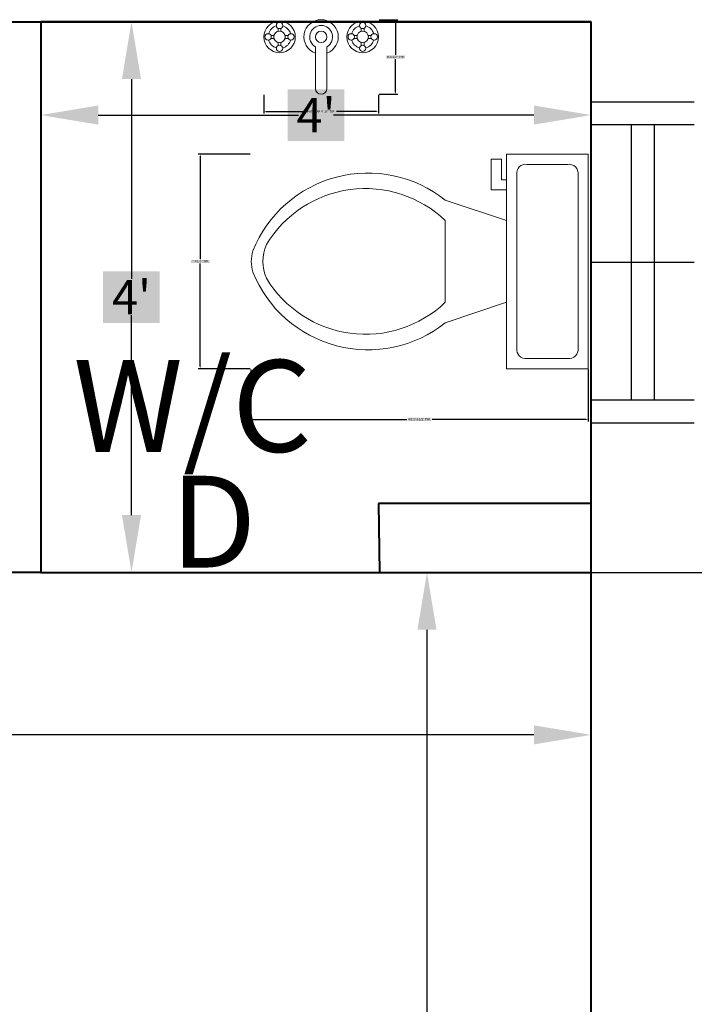
# Model space of a CAD drawing. Units: inches. Extents: x -301 to 715, y -607 to 364.
# Tile 93 of 141: x 74 to 133, y -168 to -83. Entities that reach past the tile are written whole.
import ezdxf

# ---------------------------------------------------------------- set-up
doc = ezdxf.new("R2010")
doc.units = ezdxf.units.IN
doc.header["$MEASUREMENT"] = 0
for name, color, linetype, lineweight in [('A-ANNO-DIMS', 2, 'Continuous', 18), ('A-ANNO-TEXT', 4, 'Continuous', 18), ('A-AREA-IDEN', 220, 'Continuous', 25), ('A-FLOR-FIXT', 9, 'Continuous', 18), ('A-GLAZ', 2, 'Continuous', 25), ('A-WALL', 3, 'Continuous', 40)]:
    doc.layers.add(name, color=color, linetype=linetype, lineweight=lineweight)
doc.styles.get("Standard").update_dxf_attribs({"font": 'arial.ttf'})
doc.dimstyles.get("Standard").update_dxf_attribs({"dimtxt": 0.18, "dimasz": 0.18, "dimexe": 0.18, "dimexo": 0.0625, "dimgap": 0.09, "dimtad": 0, "dimtih": 1, "dimtoh": 1, "dimdec": 1, "dimzin": 0, "dimdsep": 46, "dimlunit": 4, "dimtxsty": 'Standard', "dimcen": 0.09, "dimclrd": 3, "dimclre": 4, "dimclrt": 6, "dimadec": 0, "dimazin": 0, "dimtfac": 1, "dimtdec": 1, "dimtofl": 0, "dimtmove": 0, "dimatfit": 3, "dimfxl": 1, "dimtfill": 2, "dimtfillclr": 51, "dimtolj": 1, "dimtzin": 0, "dimarcsym": 0})

# ---------------------------------------------------------------- blocks, each defined once
blk = doc.blocks.new('Toilet - top')
for p, q in [((9.5, -6), (9.5, -2)), ((-10, -8.5), (-8, -8.5)), ((-10, -9.5), (-10, -8.5)), ((-8, -8.5), (-8, -8)), ((-7, -8), (-7, -9.5)), ((-4, -8), (-6, -14)), ((4, -8), (6, -14)), ((-7, -9.5), (-10, -9.5)), ((4, -14), (-4, -14))]:
    blk.add_line(p, q)
blk.add_lwpolyline([(10.5, -8), (10.5, 0), (-10.5, 0), (-10.5, -8)], close=True)
for points in [[(8.5, -1), (-8.5, -1)], [(-9.5, -2), (-9.5, -6)], [(-8.5, -7), (8.5, -7)]]:
    blk.add_lwpolyline(points)
for centre, radius, start, end in [((-8.625, -1.875), 0.884, 81.8699, 188.1301), ((8.625, -1.875), 0.884, 351.8699, 98.1301), ((-8.625, -6.125), 0.884, 171.8699, 278.1301), ((8.625, -6.125), 0.884, 261.8699, 8.1301), ((3.52, -21.58), 12.169, 141.46911, 247.97143), ((4.2, -21.817), 11.329, 136.36773, 238.94682), ((-3.519, -21.58), 12.169, 292.02843, 38.53071), ((-4.2, -21.817), 11.329, 301.05301, 43.63209), ((0, -27.876), 4, 245.73182, 294.26817), ((0, -29), 4, 254.86053, 285.13947)]:
    blk.add_arc(centre, radius, start, end)
blk = doc.blocks.new('Faucet - Bathroom top')
for p, q in [((-4.107, 0.125), (-4.375, 0.125)), ((-3.75, 0.4788), (-3.75, 0.75)), ((-3.5, 0.482), (-3.5, 0.75)), ((-3.1461, 0.125), (-2.875, 0.125)), ((3.143, 0.125), (2.875, 0.125)), ((3.5, 0.4788), (3.5, 0.75)), ((3.75, 0.482), (3.75, 0.75)), ((4.1039, 0.125), (4.375, 0.125)), ((-4.1039, -0.125), (-4.375, -0.125)), ((-3.75, -0.4821), (-3.75, -0.75)), ((-3.5, -0.4789), (-3.5, -0.75)), ((-3.143, -0.125), (-2.875, -0.125)), ((3.1461, -0.125), (2.875, -0.125)), ((3.5, -0.4821), (3.5, -0.75)), ((3.75, -0.4789), (3.75, -0.75)), ((4.107, -0.125), (4.375, -0.125)), ((-0.5, -0.8639), (-0.5, -4.5)), ((0.5, -4.5), (0.5, -0.8631))]:
    blk.add_line(p, q)
for centre, radius in [((-3.625, 0), 1.375), ((-3.625, 1), 0.2795), ((3.625, 0), 1.375), ((3.625, 1), 0.2795), ((-4.625, 0), 0.2795), ((-3.625, 0), 0.5), ((-2.625, 0), 0.2795), ((0, 0), 0.5), ((2.625, 0), 0.2795), ((3.625, 0), 0.5), ((4.625, 0), 0.2795), ((-3.625, -1), 0.2795), ((3.625, -1), 0.2795)]:
    blk.add_circle(centre, radius)
for centre, radius, start, end in [((-3.625, 0), 1, 105.2407, 164.2093), ((-3.625, 0), 1, 16.44125, 74.07887), ((0, 0), 1.5, 289.6514, 250.3603), ((0, 0), 1, 300.3431, 239.7554), ((3.625, 0), 1, 106.12, 164.0884), ((3.625, 0), 1, 16.23422, 73.90469), ((-3.625, 0), 1, 196.2342, 253.9047), ((-3.625, 0), 1, 286.12, 344.0884), ((3.625, 0), 1, 196.4413, 254.0789), ((3.625, 0), 1, 285.2407, 344.2093), ((0, -4.5), 0.5, 180, 0)]:
    blk.add_arc(centre, radius, start, end)
blk = doc.blocks.new('*D42')
at = {"layer": 'A-ANNO-DIMS', "color": 0, "lineweight": -2, "transparency": 16777216}
for p, q in [((-45.603, -130.88), (-45.603, -145.164)), ((123.897, -130.88), (123.897, -145.164)), ((-40.603, -144.984), (32.951, -144.984)), ((118.897, -144.984), (45.342, -144.984))]:
    blk.add_line(p, q, dxfattribs=at)
at = {"layer": 'A-ANNO-DIMS', "color": 0, "transparency": 16777216}
for points in [[(-40.603, -144.151), (-40.603, -145.818), (-45.603, -144.984)], [(118.897, -144.151), (118.897, -145.818), (123.897, -144.984)]]:
    blk.add_solid(points, dxfattribs=at)
at = {"layer": 'Defpoints', "color": 0, "transparency": 16777216}
for p in [(-45.603, -130.818), (123.897, -130.818), (-45.603, -144.984)]:
    blk.add_point(p, dxfattribs=at)
at = {"layer": 'A-ANNO-DIMS', "color": 0, "transparency": 16777216, "insert": (39.147, -144.984), "char_height": 3, "attachment_point": 5, "bg_fill": 1, "box_fill_scale": 1.25, "bg_fill_color": 51, "bg_fill_transparency": 0}
blk.add_mtext('\\A1;14\'-1{\\H1x;\\S1/2;}"', dxfattribs=at)
blk = doc.blocks.new('*D43')
at = {"layer": 'A-ANNO-DIMS', "color": 0, "lineweight": -2, "transparency": 16777216}
for p, q in [((123.834, -130.818), (109.393, -130.818)), ((109.573, -135.818), (109.573, -171.228)), ((109.573, -209.818), (109.573, -174.408)), ((123.834, -214.818), (109.393, -214.818))]:
    blk.add_line(p, q, dxfattribs=at)
at = {"layer": 'A-ANNO-DIMS', "color": 0, "transparency": 16777216}
for points in [[(108.739, -135.818), (110.406, -135.818), (109.573, -130.818)], [(108.739, -209.818), (110.406, -209.818), (109.573, -214.818)]]:
    blk.add_solid(points, dxfattribs=at)
at = {"layer": 'Defpoints', "color": 0, "transparency": 16777216}
for p in [(123.897, -130.818), (109.573, -214.818), (123.897, -214.818)]:
    blk.add_point(p, dxfattribs=at)
at = {"layer": 'A-ANNO-DIMS', "color": 0, "transparency": 16777216, "insert": (109.573, -172.818), "char_height": 3, "attachment_point": 5, "bg_fill": 1, "box_fill_scale": 1.25, "bg_fill_color": 51, "bg_fill_transparency": 0}
blk.add_mtext("\\A1;7'", dxfattribs=at)
blk = doc.blocks.new('*D44')
at = {"layer": 'A-ANNO-DIMS', "color": 0, "lineweight": -2, "transparency": 16777216}
for p, q in [((75.897, -82.88), (75.897, -91.136)), ((123.897, -82.88), (123.897, -91.136)), ((80.897, -90.956), (98.366, -90.956)), ((118.897, -90.956), (101.427, -90.956))]:
    blk.add_line(p, q, dxfattribs=at)
at = {"layer": 'A-ANNO-DIMS', "color": 0, "transparency": 16777216}
for points in [[(80.897, -90.122), (80.897, -91.789), (75.897, -90.956)], [(118.897, -90.122), (118.897, -91.789), (123.897, -90.956)]]:
    blk.add_solid(points, dxfattribs=at)
at = {"layer": 'Defpoints', "color": 0, "transparency": 16777216}
for p in [(75.897, -82.818), (123.897, -82.818), (123.897, -90.956)]:
    blk.add_point(p, dxfattribs=at)
at = {"layer": 'A-ANNO-DIMS', "color": 0, "transparency": 16777216, "insert": (99.897, -90.956), "char_height": 3, "attachment_point": 5, "bg_fill": 1, "box_fill_scale": 1.25, "bg_fill_color": 51, "bg_fill_transparency": 0}
blk.add_mtext("\\A1;4'", dxfattribs=at)
blk = doc.blocks.new('*D45')
at = {"layer": 'A-ANNO-DIMS', "color": 0, "lineweight": -2, "transparency": 16777216}
for p, q in [((75.959, -82.818), (83.975, -82.818)), ((83.795, -87.818), (83.795, -105.228)), ((83.795, -125.818), (83.795, -108.408)), ((75.959, -130.818), (83.975, -130.818))]:
    blk.add_line(p, q, dxfattribs=at)
at = {"layer": 'A-ANNO-DIMS', "color": 0, "transparency": 16777216}
for points in [[(82.961, -87.818), (84.628, -87.818), (83.795, -82.818)], [(82.961, -125.818), (84.628, -125.818), (83.795, -130.818)]]:
    blk.add_solid(points, dxfattribs=at)
at = {"layer": 'Defpoints', "color": 0, "transparency": 16777216}
for p in [(75.897, -82.818), (75.897, -130.818), (83.795, -130.818)]:
    blk.add_point(p, dxfattribs=at)
at = {"layer": 'A-ANNO-DIMS', "color": 0, "transparency": 16777216, "insert": (83.795, -106.818), "char_height": 3, "attachment_point": 5, "bg_fill": 1, "box_fill_scale": 1.25, "bg_fill_color": 51, "bg_fill_transparency": 0}
blk.add_mtext("\\A1;4'", dxfattribs=at)
blk = doc.blocks.new('VENT-24-PLAN')
for p, q in [((0, 0), (0, 9)), ((2, 0), (2, 9)), ((14, 0), (14, 9)), ((26, 0), (26, 9)), ((28, 0), (28, 9)), ((26, 5.5), (2, 5.5)), ((26, 3.5), (2, 3.5))]:
    blk.add_line(p, q)
blk = doc.blocks.new('*D110')
at = {"layer": 'A-ANNO-DIMS', "color": 4, "lineweight": -2, "transparency": 16777216}
for p, q in [((94.208, -113.126), (94.208, -117.659)), ((123.642, -113.126), (123.642, -117.659))]:
    blk.add_line(p, q, dxfattribs=at)
at = {"layer": 'A-ANNO-DIMS', "color": 3, "lineweight": -2, "transparency": 16777216}
for p, q in [((94.388, -117.479), (107.829, -117.479)), ((123.462, -117.479), (110.021, -117.479))]:
    blk.add_line(p, q, dxfattribs=at)
at = {"layer": 'A-ANNO-DIMS', "color": 3, "transparency": 16777216}
for points in [[(94.388, -117.449), (94.388, -117.509), (94.208, -117.479)], [(123.462, -117.449), (123.462, -117.509), (123.642, -117.479)]]:
    blk.add_solid(points, dxfattribs=at)
at = {"layer": 'Defpoints', "color": 0, "transparency": 16777216}
for p in [(94.208, -113.064), (123.642, -113.064), (123.642, -117.479)]:
    blk.add_point(p, dxfattribs=at)
at = {"layer": 'A-ANNO-DIMS', "color": 6, "transparency": 16777216, "insert": (108.925, -117.479), "char_height": 0.18, "attachment_point": 5, "bg_fill": 1, "box_fill_scale": 1.25, "bg_fill_color": 51, "bg_fill_transparency": 0}
blk.add_mtext('\\A1;WC 2\'-5 1/2" TYP.', dxfattribs=at)
blk = doc.blocks.new('*D111')
at = {"layer": 'A-ANNO-DIMS', "color": 4, "lineweight": -2, "transparency": 16777216}
for p, q in [((94.146, -94.36), (89.613, -94.36)), ((94.146, -113.064), (89.613, -113.064))]:
    blk.add_line(p, q, dxfattribs=at)
at = {"layer": 'A-ANNO-DIMS', "color": 3, "lineweight": -2, "transparency": 16777216}
for p, q in [((89.793, -94.54), (89.793, -103.529)), ((89.793, -112.884), (89.793, -103.895))]:
    blk.add_line(p, q, dxfattribs=at)
at = {"layer": 'A-ANNO-DIMS', "color": 3, "transparency": 16777216}
for points in [[(89.763, -94.54), (89.823, -94.54), (89.793, -94.36)], [(89.763, -112.884), (89.823, -112.884), (89.793, -113.064)]]:
    blk.add_solid(points, dxfattribs=at)
at = {"layer": 'Defpoints', "color": 0, "transparency": 16777216}
for p in [(94.208, -94.36), (89.793, -113.064), (94.208, -113.064)]:
    blk.add_point(p, dxfattribs=at)
at = {"layer": 'A-ANNO-DIMS', "color": 6, "transparency": 16777216, "insert": (89.793, -103.712), "char_height": 0.18, "attachment_point": 5, "bg_fill": 1, "box_fill_scale": 1.25, "bg_fill_color": 51, "bg_fill_transparency": 0}
blk.add_mtext('\\A1;1\'-6 1/2" TYP.', dxfattribs=at)
blk = doc.blocks.new('*D112')
at = {"layer": 'A-ANNO-DIMS', "color": 4, "lineweight": -2, "transparency": 16777216}
for p, q in [((95.338, -89.203), (95.338, -90.821)), ((105.338, -89.203), (105.338, -90.821))]:
    blk.add_line(p, q, dxfattribs=at)
at = {"layer": 'A-ANNO-DIMS', "color": 3, "lineweight": -2, "transparency": 16777216}
for p, q in [((95.518, -90.641), (98.984, -90.641)), ((105.158, -90.641), (101.693, -90.641))]:
    blk.add_line(p, q, dxfattribs=at)
at = {"layer": 'A-ANNO-DIMS', "color": 3, "transparency": 16777216}
for points in [[(95.518, -90.611), (95.518, -90.671), (95.338, -90.641)], [(105.158, -90.611), (105.158, -90.671), (105.338, -90.641)]]:
    blk.add_solid(points, dxfattribs=at)
at = {"layer": 'Defpoints', "color": 0, "transparency": 16777216}
for p in [(95.338, -89.141), (105.338, -89.141), (105.338, -90.641)]:
    blk.add_point(p, dxfattribs=at)
at = {"layer": 'A-ANNO-DIMS', "color": 6, "transparency": 16777216, "insert": (100.338, -90.641), "char_height": 0.18, "attachment_point": 5, "bg_fill": 1, "box_fill_scale": 1.25, "bg_fill_color": 51, "bg_fill_transparency": 0}
blk.add_mtext('\\A1;BATH TAP 0\'-10" TYP.', dxfattribs=at)
blk = doc.blocks.new('*D113')
at = {"layer": 'A-ANNO-DIMS', "color": 4, "lineweight": -2, "transparency": 16777216}
for p, q in [((105.401, -82.641), (107.018, -82.641)), ((105.401, -89.141), (107.018, -89.141))]:
    blk.add_line(p, q, dxfattribs=at)
at = {"layer": 'A-ANNO-DIMS', "color": 3, "lineweight": -2, "transparency": 16777216}
for p, q in [((106.838, -82.821), (106.838, -85.708)), ((106.838, -88.961), (106.838, -86.074))]:
    blk.add_line(p, q, dxfattribs=at)
at = {"layer": 'A-ANNO-DIMS', "color": 3, "transparency": 16777216}
for points in [[(106.808, -82.821), (106.868, -82.821), (106.838, -82.641)], [(106.808, -88.961), (106.868, -88.961), (106.838, -89.141)]]:
    blk.add_solid(points, dxfattribs=at)
at = {"layer": 'Defpoints', "color": 0, "transparency": 16777216}
for p in [(105.338, -82.641), (106.838, -82.641), (105.338, -89.141)]:
    blk.add_point(p, dxfattribs=at)
at = {"layer": 'A-ANNO-DIMS', "color": 6, "transparency": 16777216, "insert": (106.838, -85.891), "char_height": 0.18, "attachment_point": 5, "bg_fill": 1, "box_fill_scale": 1.25, "bg_fill_color": 51, "bg_fill_transparency": 0}
blk.add_mtext('\\A1;0\'-6 1/2" TYP.', dxfattribs=at)
blk = doc.blocks.new('*D152')
at = {"layer": 'A-ANNO-DIMS', "color": 4, "lineweight": -2, "transparency": 16777216}
for p, q in [((123.959, -130.818), (233.659, -130.818)), ((132.959, -223.818), (233.659, -223.818))]:
    blk.add_line(p, q, dxfattribs=at)
at = {"layer": 'A-ANNO-DIMS', "color": 3, "lineweight": -2, "transparency": 16777216}
for p, q in [((233.479, -130.998), (233.479, -177.136)), ((233.479, -223.638), (233.479, -177.5))]:
    blk.add_line(p, q, dxfattribs=at)
at = {"layer": 'A-ANNO-DIMS', "color": 3, "transparency": 16777216}
for points in [[(233.449, -130.998), (233.509, -130.998), (233.479, -130.818)], [(233.449, -223.638), (233.509, -223.638), (233.479, -223.818)]]:
    blk.add_solid(points, dxfattribs=at)
at = {"layer": 'Defpoints', "color": 0, "transparency": 16777216}
for p in [(123.897, -130.818), (233.479, -130.818), (132.897, -223.818)]:
    blk.add_point(p, dxfattribs=at)
at = {"layer": 'A-ANNO-DIMS', "color": 6, "transparency": 16777216, "insert": (233.479, -177.318), "char_height": 0.18, "attachment_point": 5, "bg_fill": 1, "box_fill_scale": 1.25, "bg_fill_color": 51, "bg_fill_transparency": 0}
blk.add_mtext('\\A1;7\'-9"', dxfattribs=at)

msp = doc.modelspace()

# ---------------------------------------------------------------- linework, layer by layer
at = {"layer": 'A-WALL'}
for p, q in [((57.161, -82.818), (123.897, -82.818)), ((123.897, -82.818), (75.897, -82.818)), ((75.897, -82.818), (75.897, -130.818)), ((123.897, -214.818), (123.897, -82.818)), ((123.897, -124.818), (105.352, -124.818)), ((105.352, -124.818), (105.424, -130.818)), ((75.897, -130.818), (21.897, -130.818)), ((75.897, -130.818), (105.424, -130.818)), ((104.088, -130.818), (123.897, -130.818))]:
    msp.add_line(p, q, dxfattribs=at)

# ---------------------------------------------------------------- block references
at = {"layer": 'A-FLOR-FIXT'}
msp.add_blockref('Faucet - Bathroom top', (100.338, -84.141), dxfattribs=at)
at = {"layer": 'A-FLOR-FIXT', "xscale": 0.8906747211908207, "yscale": 0.8906747211908207, "zscale": 0.8906747211908207, "rotation": 270}
msp.add_blockref('Toilet - top', (123.642, -103.712), dxfattribs=at)
at = {"layer": 'A-GLAZ', "rotation": 89.99999999999957}
msp.add_blockref('VENT-24-PLAN', (132.897, -117.818), dxfattribs=at)

# ---------------------------------------------------------------- texts
at = {"layer": 'A-ANNO-TEXT'}
msp.add_text('D', height=8, dxfattribs=at).set_placement((87.181, -130.401))
at = {"layer": 'A-AREA-IDEN', "insert": (78.709, -112.312), "char_height": 8, "attachment_point": 1}
msp.add_mtext_dynamic_manual_height_columns('W/C', width=73.06001, gutter_width=1, heights=[0], dxfattribs=at)

# ---------------------------------------------------------------- dimensions: what is measured, and where the dimension line sits
at = {"layer": 'A-ANNO-DIMS'}
for base, p1, p2, picture, middle in [((123.897, -90.956), (75.897, -82.818), (123.897, -82.818), '*D44', (99.897, -90.956)), ((-45.603, -144.984), (123.897, -130.818), (-45.603, -130.818), '*D42', (39.147, -144.984))]:
    dim = msp.add_linear_dim(base=base, p1=p1, p2=p2, dimstyle='Standard', override={"dimtxt": 3, "dimasz": 5, "dimclrd": 0, "dimclre": 0, "dimclrt": 0}, dxfattribs=at)
    dim.commit()
    dim.dimension.update_dxf_attribs({"geometry": picture, "text_midpoint": middle})
for base, p1, p2, override, picture, middle in [((83.795, -130.818), (75.897, -82.818), (75.897, -130.818), {"dimtxt": 3, "dimasz": 5, "dimclrd": 0, "dimclre": 0, "dimclrt": 0}, '*D45', (83.795, -106.818)), ((109.573, -214.818), (123.897, -130.818), (123.897, -214.818), {"dimtxt": 3, "dimasz": 5, "dimclrd": 0, "dimclre": 0, "dimclrt": 0}, '*D43', (109.573, -172.818)), ((233.479, -130.818), (132.897, -223.818), (123.897, -130.818), {"dimdec": 1, "dimlfac": 1, "dimrnd": 0, "dimzin": 1, "dimdsep": 46, "dimlunit": 4, "dimfrac": 2}, '*D152', (233.479, -177.318))]:
    dim = msp.add_linear_dim(base=base, p1=p1, p2=p2, angle=90, dimstyle='Standard', override=override, dxfattribs=at)
    dim.commit()
    dim.dimension.update_dxf_attribs({"geometry": picture, "text_midpoint": middle})
for base, p1, p2, angle, picture, middle in [((106.838, -82.641), (105.338, -89.141), (105.338, -82.641), 90, '*D113', (106.838, -85.891)), ((89.793, -113.064), (94.208, -94.36), (94.208, -113.064), 270, '*D111', (89.793, -103.712))]:
    dim = msp.add_linear_dim(base=base, p1=p1, p2=p2, angle=angle, text='<> TYP.', dimstyle='Standard', override={"dimdec": 1, "dimlfac": 1, "dimrnd": 0, "dimzin": 1, "dimdsep": 46, "dimlunit": 4, "dimfrac": 2}, dxfattribs=at)
    dim.commit()
    dim.dimension.update_dxf_attribs({"geometry": picture, "text_midpoint": middle})
for base, p1, p2, text, picture, middle in [((105.338, -90.641), (95.338, -89.141), (105.338, -89.141), 'BATH TAP <> TYP.', '*D112', (100.338, -90.641)), ((123.642, -117.479), (94.208, -113.064), (123.642, -113.064), 'WC <> TYP.', '*D110', (108.925, -117.479))]:
    dim = msp.add_linear_dim(base=base, p1=p1, p2=p2, text=text, dimstyle='Standard', override={"dimdec": 1, "dimlfac": 1, "dimrnd": 0, "dimzin": 1, "dimdsep": 46, "dimlunit": 4, "dimfrac": 2}, dxfattribs=at)
    dim.commit()
    dim.dimension.update_dxf_attribs({"geometry": picture, "text_midpoint": middle})

doc.saveas('drawing.dxf')
